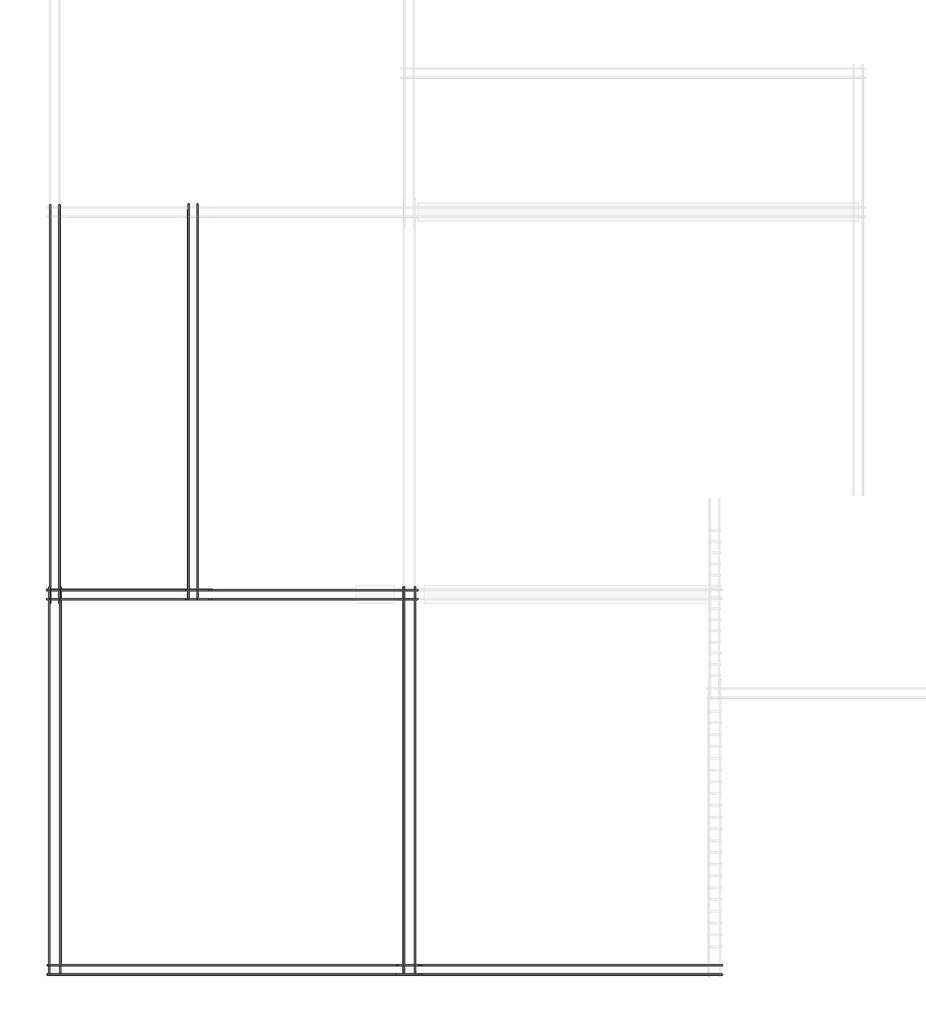
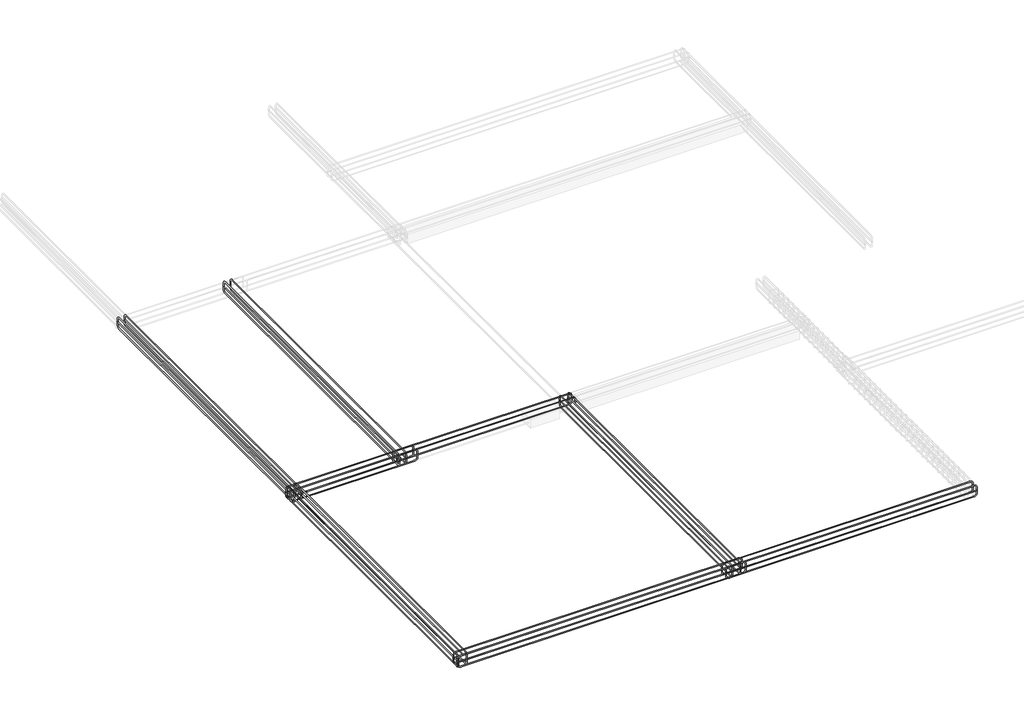
# One storey, part 2 of 5: 45 reinforcing bars.
"""IFC4 building model written with IfcOpenShell, lengths in millimetres."""

from ifc_helpers import new_model, si_unit, point, frame, origin, place, context, project, spatial, polyline, circle_curve, trimmed, segment, composite_curve, element, save
from ifc_brep_helpers import swept_disk

model = new_model("IFC4")

# Units and contexts
model_context = context("Model", 3, world=origin())
ifc_project = project(units=[si_unit("LENGTHUNIT", "METRE", prefix="MILLI")], contexts=[model_context])

# Site, building, storey
site = spatial("IfcSite", under=ifc_project)
building = spatial("IfcBuilding", under=site)
storey = spatial("IfcBuildingStorey", under=building, Elevation=0.0)

# Reinforcing bars
placement = place(None, origin())
element("IfcReinforcingBar", 1, at=placement, inside=storey, context=model_context, shape_type="SolidModel", body=[
    swept_disk(composite_curve([segment(polyline([(-14810.5016244, 4871.519882, 304.2552561), (-14810.5016244, 4871.519882, 355.0552561)]), True, "CONTINUOUS"), segment(trimmed(circle_curve(frame((-14766.0516244, 4871.519882, 355.0552561), z_axis=(0.0, 1.0, 0.0), x_axis=(-44.45000000000073, 0.0, 0.0)), 44.45), [point((-14810.5016244, 4871.519882, 355.0552561))], [point((-14766.0516244, 4871.519882, 399.5052561))], True, "CARTESIAN"), True, "CONTINUOUS"), segment(polyline([(-14766.0516244, 4871.519882, 399.5052561), (-12753.7926107, 4871.519882, 399.5052561)]), True, "CONTINUOUS"), segment(trimmed(circle_curve(frame((-12753.7926107, 4871.519882, 355.0552561), z_axis=(0.0, 1.0, 0.0), x_axis=(0.0, 0.0, 44.44999999999999)), 44.45), [point((-12753.7926107, 4871.519882, 399.5052561))], [point((-12709.3426107, 4871.519882, 355.0552561))], True, "CARTESIAN"), True, "CONTINUOUS"), segment(polyline([(-12709.3426107, 4871.519882, 355.0552561), (-12709.3426107, 4871.519882, 304.2552561)]), True, "CONTINUOUS")], self_intersect=False), 6.35),
])
element("IfcReinforcingBar", 2, at=placement, inside=storey, context=model_context, shape_type="SolidModel", body=[
    swept_disk(composite_curve([segment(polyline([(-14811.119206, 4984.7303943, 304.2552561), (-14811.119206, 4984.7303943, 355.0552561)]), True, "CONTINUOUS"), segment(trimmed(circle_curve(frame((-14766.669206, 4984.7303943, 355.0552561), z_axis=(0.0, 1.0, 0.0), x_axis=(-44.44999999999891, 0.0, 0.0)), 44.45), [point((-14811.119206, 4984.7303943, 355.0552561))], [point((-14766.669206, 4984.7303943, 399.5052561))], True, "CARTESIAN"), True, "CONTINUOUS"), segment(polyline([(-14766.669206, 4984.7303943, 399.5052561), (-12753.8888906, 4984.7303943, 399.5052561)]), True, "CONTINUOUS"), segment(trimmed(circle_curve(frame((-12753.8888906, 4984.7303943, 355.0552561), z_axis=(0.0, 1.0, 0.0), x_axis=(0.0, 0.0, 44.44999999999999)), 44.45), [point((-12753.8888906, 4984.7303943, 399.5052561))], [point((-12709.4388906, 4984.7303943, 355.0552561))], True, "CARTESIAN"), True, "CONTINUOUS"), segment(polyline([(-12709.4388906, 4984.7303943, 355.0552561), (-12709.4388906, 4984.7303943, 304.2552561)]), True, "CONTINUOUS")], self_intersect=False), 6.35),
])
element("IfcReinforcingBar", 3, at=placement, inside=storey, context=model_context, shape_type="SolidModel", body=[
    swept_disk(composite_curve([segment(polyline([(-14810.6974131, 4871.519882, 305.3447439), (-14810.6974131, 4871.519882, 254.5447439)]), True, "CONTINUOUS"), segment(trimmed(circle_curve(frame((-14766.2474131, 4871.519882, 254.5447439), z_axis=(0.0, -1.0, 0.0), x_axis=(-44.45000000000073, 0.0, 0.0)), 44.45), [point((-14810.6974131, 4871.519882, 254.5447439))], [point((-14766.2474131, 4871.519882, 210.0947439))], True, "CARTESIAN"), True, "CONTINUOUS"), segment(polyline([(-14766.2474131, 4871.519882, 210.0947439), (-12754.044612, 4871.519882, 210.0947439)]), True, "CONTINUOUS"), segment(trimmed(circle_curve(frame((-12754.044612, 4871.519882, 254.5447439), z_axis=(0.0, -1.0, 0.0), x_axis=(0.0, 0.0, -44.44999999999999)), 44.45), [point((-12754.044612, 4871.519882, 210.0947439))], [point((-12709.594612, 4871.519882, 254.5447439))], True, "CARTESIAN"), True, "CONTINUOUS"), segment(polyline([(-12709.594612, 4871.519882, 254.5447439), (-12709.594612, 4871.519882, 305.3447439)]), True, "CONTINUOUS")], self_intersect=False), 6.35),
])
element("IfcReinforcingBar", 4, at=placement, inside=storey, context=model_context, shape_type="SolidModel", body=[
    swept_disk(composite_curve([segment(polyline([(-14812.0419124, 4984.7303943, 305.3447439), (-14812.0419124, 4984.7303943, 254.5447439)]), True, "CONTINUOUS"), segment(trimmed(circle_curve(frame((-14767.5919124, 4984.7303943, 254.5447439), z_axis=(0.0, -1.0, 0.0), x_axis=(-44.45000000000073, 0.0, 0.0)), 44.45), [point((-14812.0419124, 4984.7303943, 254.5447439))], [point((-14767.5919124, 4984.7303943, 210.0947439))], True, "CARTESIAN"), True, "CONTINUOUS"), segment(polyline([(-14767.5919124, 4984.7303943, 210.0947439), (-12754.4128441, 4984.7303943, 210.0947439)]), True, "CONTINUOUS"), segment(trimmed(circle_curve(frame((-12754.4128441, 4984.7303943, 254.5447439), z_axis=(0.0, -1.0, 0.0), x_axis=(0.0, 0.0, -44.44999999999999)), 44.45), [point((-12754.4128441, 4984.7303943, 210.0947439))], [point((-12709.9628441, 4984.7303943, 254.5447439))], True, "CARTESIAN"), True, "CONTINUOUS"), segment(polyline([(-12709.9628441, 4984.7303943, 254.5447439), (-12709.9628441, 4984.7303943, 305.3447439)]), True, "CONTINUOUS")], self_intersect=False), 6.35),
])
element("IfcReinforcingBar", 5, at=placement, inside=storey, context=model_context, shape_type="SolidModel", body=[
    swept_disk(composite_curve([segment(polyline([(-14534.7918223, 4867.8001382, 304.8), (-13131.4418223, 4867.8001382, 304.8)]), True, "CONTINUOUS")], self_intersect=False), 6.35),
])
element("IfcReinforcingBar", 6, at=placement, inside=storey, context=model_context, shape_type="SolidModel", body=[
    swept_disk(composite_curve([segment(polyline([(-14818.480298, 4988.4501382, 304.8), (-12703.1933611, 4988.4501382, 304.8)]), True, "CONTINUOUS")], self_intersect=False), 6.35),
])
element("IfcReinforcingBar", 7, at=placement, inside=storey, context=model_context, shape_type="SolidModel", body=[
    swept_disk(composite_curve([segment(polyline([(-10097.104427, 4984.7303943, 304.2552561), (-10097.104427, 4984.7303943, 355.0552561)]), True, "CONTINUOUS"), segment(trimmed(circle_curve(frame((-10141.554427, 4984.7303943, 355.0552561), z_axis=(0.0, -1.0, 0.0), x_axis=(44.44999999999891, 0.0, 0.0)), 44.45), [point((-10097.104427, 4984.7303943, 355.0552561))], [point((-10141.554427, 4984.7303943, 399.5052561))], True, "CARTESIAN"), True, "CONTINUOUS"), segment(polyline([(-10141.554427, 4984.7303943, 399.5052561), (-13001.0910339, 4984.7303943, 399.5052561)]), True, "CONTINUOUS"), segment(trimmed(circle_curve(frame((-13001.0910339, 4984.7303943, 355.0552561), z_axis=(0.0, -1.0, 0.0), x_axis=(0.0, 0.0, 44.44999999999999)), 44.45), [point((-13001.0910339, 4984.7303943, 399.5052561))], [point((-13045.5410339, 4984.7303943, 355.0552561))], True, "CARTESIAN"), True, "CONTINUOUS"), segment(polyline([(-13045.5410339, 4984.7303943, 355.0552561), (-13045.5410339, 4984.7303943, 304.2552561)]), True, "CONTINUOUS")], self_intersect=False), 6.35),
])
element("IfcReinforcingBar", 8, at=placement, inside=storey, context=model_context, shape_type="SolidModel", body=[
    swept_disk(composite_curve([segment(polyline([(-10097.5426731, 4871.519882, 304.2552561), (-10097.5426731, 4871.519882, 355.0552561)]), True, "CONTINUOUS"), segment(trimmed(circle_curve(frame((-10141.9926731, 4871.519882, 355.0552561), z_axis=(0.0, -1.0, 0.0), x_axis=(44.44999999999891, 0.0, 0.0)), 44.45), [point((-10097.5426731, 4871.519882, 355.0552561))], [point((-10141.9926731, 4871.519882, 399.5052561))], True, "CARTESIAN"), True, "CONTINUOUS"), segment(polyline([(-10141.9926731, 4871.519882, 399.5052561), (-13000.994754, 4871.519882, 399.5052561)]), True, "CONTINUOUS"), segment(trimmed(circle_curve(frame((-13000.994754, 4871.519882, 355.0552561), z_axis=(0.0, -1.0, 0.0), x_axis=(0.0, 0.0, 44.44999999999999)), 44.45), [point((-13000.994754, 4871.519882, 399.5052561))], [point((-13045.444754, 4871.519882, 355.0552561))], True, "CARTESIAN"), True, "CONTINUOUS"), segment(polyline([(-13045.444754, 4871.519882, 355.0552561), (-13045.444754, 4871.519882, 304.2552561)]), True, "CONTINUOUS")], self_intersect=False), 6.35),
])
element("IfcReinforcingBar", 9, at=placement, inside=storey, context=model_context, shape_type="SolidModel", body=[
    swept_disk(composite_curve([segment(polyline([(-10095.8402778, 4984.7303943, 305.3447439), (-10095.8402778, 4984.7303943, 254.5447439)]), True, "CONTINUOUS"), segment(trimmed(circle_curve(frame((-10140.2902778, 4984.7303943, 254.5447439), z_axis=(0.0, 1.0, 0.0), x_axis=(44.45000000000073, 0.0, 0.0)), 44.45), [point((-10095.8402778, 4984.7303943, 254.5447439))], [point((-10140.2902778, 4984.7303943, 210.0947439))], True, "CARTESIAN"), True, "CONTINUOUS"), segment(polyline([(-10140.2902778, 4984.7303943, 210.0947439), (-13000.8390327, 4984.7303943, 210.0947439)]), True, "CONTINUOUS"), segment(trimmed(circle_curve(frame((-13000.8390327, 4984.7303943, 254.5447439), z_axis=(0.0, 1.0, 0.0), x_axis=(0.0, 0.0, -44.44999999999999)), 44.45), [point((-13000.8390327, 4984.7303943, 210.0947439))], [point((-13045.2890327, 4984.7303943, 254.5447439))], True, "CARTESIAN"), True, "CONTINUOUS"), segment(polyline([(-13045.2890327, 4984.7303943, 254.5447439), (-13045.2890327, 4984.7303943, 305.3447439)]), True, "CONTINUOUS")], self_intersect=False), 6.35),
])
element("IfcReinforcingBar", 10, at=placement, inside=storey, context=model_context, shape_type="SolidModel", body=[
    swept_disk(composite_curve([segment(polyline([(-6221.7854997, 209.9629274, 304.2552561), (-6221.7854997, 209.9629274, 355.0552561)]), True, "CONTINUOUS"), segment(trimmed(circle_curve(frame((-6266.2354997, 209.9629274, 355.0552561), z_axis=(0.0, -1.0, 0.0), x_axis=(44.44999999999982, 0.0, 0.0)), 44.45), [point((-6221.7854997, 209.9629274, 355.0552561))], [point((-6266.2354997, 209.9629274, 399.5052561))], True, "CARTESIAN"), True, "CONTINUOUS"), segment(polyline([(-6266.2354997, 209.9629274, 399.5052561), (-10321.3910339, 209.9629274, 399.5052561)]), True, "CONTINUOUS"), segment(trimmed(circle_curve(frame((-10321.3910339, 209.9629274, 355.0552561), z_axis=(0.0, -1.0, 0.0), x_axis=(0.0, 0.0, 44.44999999999999)), 44.45), [point((-10321.3910339, 209.9629274, 399.5052561))], [point((-10365.8410339, 209.9629274, 355.0552561))], True, "CARTESIAN"), True, "CONTINUOUS"), segment(polyline([(-10365.8410339, 209.9629274, 355.0552561), (-10365.8410339, 209.9629274, 304.2552561)]), True, "CONTINUOUS")], self_intersect=False), 6.35),
])
element("IfcReinforcingBar", 11, at=placement, inside=storey, context=model_context, shape_type="SolidModel", body=[
    swept_disk(composite_curve([segment(polyline([(-6222.3875013, 96.7524151, 304.2552561), (-6222.3875013, 96.7524151, 355.0552561)]), True, "CONTINUOUS"), segment(trimmed(circle_curve(frame((-6266.8375013, 96.7524151, 355.0552561), z_axis=(0.0, -1.0, 0.0), x_axis=(44.45000000000073, 0.0, 0.0)), 44.45), [point((-6222.3875013, 96.7524151, 355.0552561))], [point((-6266.8375013, 96.7524151, 399.5052561))], True, "CARTESIAN"), True, "CONTINUOUS"), segment(polyline([(-6266.8375013, 96.7524151, 399.5052561), (-10321.294754, 96.7524151, 399.5052561)]), True, "CONTINUOUS"), segment(trimmed(circle_curve(frame((-10321.294754, 96.7524151, 355.0552561), z_axis=(0.0, -1.0, 0.0), x_axis=(0.0, 0.0, 44.44999999999999)), 44.45), [point((-10321.294754, 96.7524151, 399.5052561))], [point((-10365.744754, 96.7524151, 355.0552561))], True, "CARTESIAN"), True, "CONTINUOUS"), segment(polyline([(-10365.744754, 96.7524151, 355.0552561), (-10365.744754, 96.7524151, 304.2552561)]), True, "CONTINUOUS")], self_intersect=False), 6.35),
])
element("IfcReinforcingBar", 12, at=placement, inside=storey, context=model_context, shape_type="SolidModel", body=[
    swept_disk(composite_curve([segment(polyline([(-6222.9639641, 209.9629274, 305.3447439), (-6222.9639641, 209.9629274, 254.5447439)]), True, "CONTINUOUS"), segment(trimmed(circle_curve(frame((-6267.4139641, 209.9629274, 254.5447439), z_axis=(0.0, 1.0, 0.0), x_axis=(44.44999999999982, 0.0, 0.0)), 44.45), [point((-6222.9639641, 209.9629274, 254.5447439))], [point((-6267.4139641, 209.9629274, 210.0947439))], True, "CARTESIAN"), True, "CONTINUOUS"), segment(polyline([(-6267.4139641, 209.9629274, 210.0947439), (-10321.1390327, 209.9629274, 210.0947439)]), True, "CONTINUOUS"), segment(trimmed(circle_curve(frame((-10321.1390327, 209.9629274, 254.5447439), z_axis=(0.0, 1.0, 0.0), x_axis=(0.0, 0.0, -44.44999999999999)), 44.45), [point((-10321.1390327, 209.9629274, 210.0947439))], [point((-10365.5890327, 209.9629274, 254.5447439))], True, "CARTESIAN"), True, "CONTINUOUS"), segment(polyline([(-10365.5890327, 209.9629274, 254.5447439), (-10365.5890327, 209.9629274, 305.3447439)]), True, "CONTINUOUS")], self_intersect=False), 6.35),
])
element("IfcReinforcingBar", 13, at=placement, inside=storey, context=model_context, shape_type="SolidModel", body=[
    swept_disk(composite_curve([segment(polyline([(-6223.2425489, 96.7524151, 305.3447439), (-6223.2425489, 96.7524151, 254.5447439)]), True, "CONTINUOUS"), segment(trimmed(circle_curve(frame((-6267.6925489, 96.7524151, 254.5447439), z_axis=(0.0, 1.0, 0.0), x_axis=(44.44999999999982, 0.0, 0.0)), 44.45), [point((-6223.2425489, 96.7524151, 254.5447439))], [point((-6267.6925489, 96.7524151, 210.0947439))], True, "CARTESIAN"), True, "CONTINUOUS"), segment(polyline([(-6267.6925489, 96.7524151, 210.0947439), (-10320.7708006, 96.7524151, 210.0947439)]), True, "CONTINUOUS"), segment(trimmed(circle_curve(frame((-10320.7708006, 96.7524151, 254.5447439), z_axis=(0.0, 1.0, 0.0), x_axis=(0.0, 0.0, -44.44999999999999)), 44.45), [point((-10320.7708006, 96.7524151, 210.0947439))], [point((-10365.2208006, 96.7524151, 254.5447439))], True, "CARTESIAN"), True, "CONTINUOUS"), segment(polyline([(-10365.2208006, 96.7524151, 254.5447439), (-10365.2208006, 96.7524151, 305.3447439)]), True, "CONTINUOUS")], self_intersect=False), 6.35),
])
element("IfcReinforcingBar", 14, at=placement, inside=storey, context=model_context, shape_type="SolidModel", body=[
    swept_disk(composite_curve([segment(polyline([(-6216.0848989, 213.6826713, 304.8), (-10311.3420725, 213.6826713, 304.8)]), True, "CONTINUOUS")], self_intersect=False), 6.35),
])
element("IfcReinforcingBar", 15, at=placement, inside=storey, context=model_context, shape_type="SolidModel", body=[
    swept_disk(composite_curve([segment(polyline([(-6215.9707513, 93.0326713, 304.8), (-10371.9902836, 93.0326713, 304.8)]), True, "CONTINUOUS")], self_intersect=False), 6.35),
])
element("IfcReinforcingBar", 16, at=placement, inside=storey, context=model_context, shape_type="SolidModel", body=[
    swept_disk(composite_curve([segment(polyline([(-10040.6958382, 209.9629274, 304.2552561), (-10040.6958382, 209.9629274, 355.0552561)]), True, "CONTINUOUS"), segment(trimmed(circle_curve(frame((-10085.1458382, 209.9629274, 355.0552561), z_axis=(0.0, -1.0, 0.0), x_axis=(44.45000000000073, 0.0, 0.0)), 44.45), [point((-10040.6958382, 209.9629274, 355.0552561))], [point((-10085.1458382, 209.9629274, 399.5052561))], True, "CARTESIAN"), True, "CONTINUOUS"), segment(polyline([(-10085.1458382, 209.9629274, 399.5052561), (-14760.0410339, 209.9629274, 399.5052561)]), True, "CONTINUOUS"), segment(trimmed(circle_curve(frame((-14760.0410339, 209.9629274, 355.0552561), z_axis=(0.0, -1.0, 0.0), x_axis=(0.0, 0.0, 44.44999999999999)), 44.45), [point((-14760.0410339, 209.9629274, 399.5052561))], [point((-14804.4910339, 209.9629274, 355.0552561))], True, "CARTESIAN"), True, "CONTINUOUS"), segment(polyline([(-14804.4910339, 209.9629274, 355.0552561), (-14804.4910339, 209.9629274, 304.2552561)]), True, "CONTINUOUS")], self_intersect=False), 6.35),
])
element("IfcReinforcingBar", 17, at=placement, inside=storey, context=model_context, shape_type="SolidModel", body=[
    swept_disk(composite_curve([segment(polyline([(-10040.7832995, 96.7524151, 304.2552561), (-10040.7832995, 96.7524151, 355.0552561)]), True, "CONTINUOUS"), segment(trimmed(circle_curve(frame((-10085.2332995, 96.7524151, 355.0552561), z_axis=(0.0, -1.0, 0.0), x_axis=(44.44999999999891, 0.0, 0.0)), 44.45), [point((-10040.7832995, 96.7524151, 355.0552561))], [point((-10085.2332995, 96.7524151, 399.5052561))], True, "CARTESIAN"), True, "CONTINUOUS"), segment(polyline([(-10085.2332995, 96.7524151, 399.5052561), (-14759.944754, 96.7524151, 399.5052561)]), True, "CONTINUOUS"), segment(trimmed(circle_curve(frame((-14759.944754, 96.7524151, 355.0552561), z_axis=(0.0, -1.0, 0.0), x_axis=(0.0, 0.0, 44.44999999999999)), 44.45), [point((-14759.944754, 96.7524151, 399.5052561))], [point((-14804.394754, 96.7524151, 355.0552561))], True, "CARTESIAN"), True, "CONTINUOUS"), segment(polyline([(-14804.394754, 96.7524151, 355.0552561), (-14804.394754, 96.7524151, 304.2552561)]), True, "CONTINUOUS")], self_intersect=False), 6.35),
])
element("IfcReinforcingBar", 18, at=placement, inside=storey, context=model_context, shape_type="SolidModel", body=[
    swept_disk(composite_curve([segment(polyline([(-10042.0160096, 209.9629274, 305.3447439), (-10042.0160096, 209.9629274, 254.5447439)]), True, "CONTINUOUS"), segment(trimmed(circle_curve(frame((-10086.4660096, 209.9629274, 254.5447439), z_axis=(0.0, 1.0, 0.0), x_axis=(44.45000000000073, 0.0, 0.0)), 44.45), [point((-10042.0160096, 209.9629274, 254.5447439))], [point((-10086.4660096, 209.9629274, 210.0947439))], True, "CARTESIAN"), True, "CONTINUOUS"), segment(polyline([(-10086.4660096, 209.9629274, 210.0947439), (-14759.7890327, 209.9629274, 210.0947439)]), True, "CONTINUOUS"), segment(trimmed(circle_curve(frame((-14759.7890327, 209.9629274, 254.5447439), z_axis=(0.0, 1.0, 0.0), x_axis=(0.0, 0.0, -44.44999999999999)), 44.45), [point((-14759.7890327, 209.9629274, 210.0947439))], [point((-14804.2390327, 209.9629274, 254.5447439))], True, "CARTESIAN"), True, "CONTINUOUS"), segment(polyline([(-14804.2390327, 209.9629274, 254.5447439), (-14804.2390327, 209.9629274, 305.3447439)]), True, "CONTINUOUS")], self_intersect=False), 6.35),
])
element("IfcReinforcingBar", 19, at=placement, inside=storey, context=model_context, shape_type="SolidModel", body=[
    swept_disk(composite_curve([segment(polyline([(-10041.3559239, 96.7524151, 305.3447439), (-10041.3559239, 96.7524151, 254.5447439)]), True, "CONTINUOUS"), segment(trimmed(circle_curve(frame((-10085.8059239, 96.7524151, 254.5447439), z_axis=(0.0, 1.0, 0.0), x_axis=(44.44999999999891, 0.0, 0.0)), 44.45), [point((-10041.3559239, 96.7524151, 254.5447439))], [point((-10085.8059239, 96.7524151, 210.0947439))], True, "CARTESIAN"), True, "CONTINUOUS"), segment(polyline([(-10085.8059239, 96.7524151, 210.0947439), (-14759.4208006, 96.7524151, 210.0947439)]), True, "CONTINUOUS"), segment(trimmed(circle_curve(frame((-14759.4208006, 96.7524151, 254.5447439), z_axis=(0.0, 1.0, 0.0), x_axis=(0.0, 0.0, -44.44999999999999)), 44.45), [point((-14759.4208006, 96.7524151, 210.0947439))], [point((-14803.8708006, 96.7524151, 254.5447439))], True, "CARTESIAN"), True, "CONTINUOUS"), segment(polyline([(-14803.8708006, 96.7524151, 254.5447439), (-14803.8708006, 96.7524151, 305.3447439)]), True, "CONTINUOUS")], self_intersect=False), 6.35),
])
element("IfcReinforcingBar", 20, at=placement, inside=storey, context=model_context, shape_type="SolidModel", body=[
    swept_disk(composite_curve([segment(polyline([(-10084.5322341, 213.6826713, 304.8), (-14809.5352998, 213.6826713, 304.8)]), True, "CONTINUOUS")], self_intersect=False), 6.35),
])
element("IfcReinforcingBar", 21, at=placement, inside=storey, context=model_context, shape_type="SolidModel", body=[
    swept_disk(composite_curve([segment(polyline([(-10086.4986582, 93.0326713, 304.8), (-14810.6402836, 93.0326713, 304.8)]), True, "CONTINUOUS")], self_intersect=False), 6.35),
])
element("IfcReinforcingBar", 22, at=placement, inside=storey, context=model_context, shape_type="SolidModel", body=[
    swept_disk(composite_curve([segment(polyline([(-10128.4365662, 92.8452695, 304.2552561), (-10128.4365662, 92.8452695, 355.0552561)]), True, "CONTINUOUS"), segment(trimmed(circle_curve(frame((-10128.4365662, 137.2952695, 355.0552561), z_axis=(-1.0, 0.0, 0.0), x_axis=(0.0, -44.44999999999999, 0.0)), 44.45), [point((-10128.4365662, 92.8452695, 355.0552561))], [point((-10128.4365662, 137.2952695, 399.5052561))], True, "CARTESIAN"), True, "CONTINUOUS"), segment(polyline([(-10128.4365662, 137.2952695, 399.5052561), (-10128.4365662, 4977.1529731, 399.5052561)]), True, "CONTINUOUS"), segment(trimmed(circle_curve(frame((-10128.4365662, 4977.1529731, 355.0552561), z_axis=(-1.0, 0.0, 0.0), x_axis=(0.0, 0.0, 44.44999999999999)), 44.45), [point((-10128.4365662, 4977.1529731, 399.5052561))], [point((-10128.4365662, 5021.6029731, 355.0552561))], True, "CARTESIAN"), True, "CONTINUOUS"), segment(polyline([(-10128.4365662, 5021.6029731, 355.0552561), (-10128.4365662, 5021.6029731, 304.2552561)]), True, "CONTINUOUS")], self_intersect=False), 6.35),
])
element("IfcReinforcingBar", 23, at=placement, inside=storey, context=model_context, shape_type="SolidModel", body=[
    swept_disk(composite_curve([segment(polyline([(-10267.0470784, 92.9792716, 304.2552561), (-10267.0470784, 92.9792716, 355.0552561)]), True, "CONTINUOUS"), segment(trimmed(circle_curve(frame((-10267.0470784, 137.4292716, 355.0552561), z_axis=(-1.0, 0.0, 0.0), x_axis=(0.0, -44.44999999999999, 0.0)), 44.45), [point((-10267.0470784, 92.9792716, 355.0552561))], [point((-10267.0470784, 137.4292716, 399.5052561))], True, "CARTESIAN"), True, "CONTINUOUS"), segment(polyline([(-10267.0470784, 137.4292716, 399.5052561), (-10267.0470784, 4977.0498865, 399.5052561)]), True, "CONTINUOUS"), segment(trimmed(circle_curve(frame((-10267.0470784, 4977.0498865, 355.0552561), z_axis=(-1.0, 0.0, 0.0), x_axis=(0.0, 0.0, 44.44999999999999)), 44.45), [point((-10267.0470784, 4977.0498865, 399.5052561))], [point((-10267.0470784, 5021.4998865, 355.0552561))], True, "CARTESIAN"), True, "CONTINUOUS"), segment(polyline([(-10267.0470784, 5021.4998865, 355.0552561), (-10267.0470784, 5021.4998865, 304.2552561)]), True, "CONTINUOUS")], self_intersect=False), 6.35),
])
element("IfcReinforcingBar", 24, at=placement, inside=storey, context=model_context, shape_type="SolidModel", body=[
    swept_disk(composite_curve([segment(polyline([(-10128.4365662, 93.5768417, 292.6447439), (-10128.4365662, 93.5768417, 241.8447439)]), True, "CONTINUOUS"), segment(trimmed(circle_curve(frame((-10128.4365662, 138.0268417, 241.8447439), z_axis=(1.0, 0.0, 0.0), x_axis=(0.0, -44.45, 0.0)), 44.45), [point((-10128.4365662, 93.5768417, 241.8447439))], [point((-10128.4365662, 138.0268417, 197.3947439))], True, "CARTESIAN"), True, "CONTINUOUS"), segment(polyline([(-10128.4365662, 138.0268417, 197.3947439), (-10128.4365662, 4976.4997012, 197.3947439)]), True, "CONTINUOUS"), segment(trimmed(circle_curve(frame((-10128.4365662, 4976.4997012, 241.8447439), z_axis=(1.0, 0.0, 0.0), x_axis=(0.0, 0.0, -44.44999999999999)), 44.45), [point((-10128.4365662, 4976.4997012, 197.3947439))], [point((-10128.4365662, 5020.9497012, 241.8447439))], True, "CARTESIAN"), True, "CONTINUOUS"), segment(polyline([(-10128.4365662, 5020.9497012, 241.8447439), (-10128.4365662, 5020.9497012, 292.6447439)]), True, "CONTINUOUS")], self_intersect=False), 6.35),
])
element("IfcReinforcingBar", 25, at=placement, inside=storey, context=model_context, shape_type="SolidModel", body=[
    swept_disk(composite_curve([segment(polyline([(-10267.0470784, 93.8151458, 292.6447439), (-10267.0470784, 93.8151458, 241.8447439)]), True, "CONTINUOUS"), segment(trimmed(circle_curve(frame((-10267.0470784, 138.2651458, 241.8447439), z_axis=(1.0, 0.0, 0.0), x_axis=(0.0, -44.45, 0.0)), 44.45), [point((-10267.0470784, 93.8151458, 241.8447439))], [point((-10267.0470784, 138.2651458, 197.3947439))], True, "CARTESIAN"), True, "CONTINUOUS"), segment(polyline([(-10267.0470784, 138.2651458, 197.3947439), (-10267.0470784, 4976.5301582, 197.3947439)]), True, "CONTINUOUS"), segment(trimmed(circle_curve(frame((-10267.0470784, 4976.5301582, 241.8447439), z_axis=(1.0, 0.0, 0.0), x_axis=(0.0, 0.0, -44.44999999999999)), 44.45), [point((-10267.0470784, 4976.5301582, 197.3947439))], [point((-10267.0470784, 5020.9801582, 241.8447439))], True, "CARTESIAN"), True, "CONTINUOUS"), segment(polyline([(-10267.0470784, 5020.9801582, 241.8447439), (-10267.0470784, 5020.9801582, 292.6447439)]), True, "CONTINUOUS")], self_intersect=False), 6.35),
])
element("IfcReinforcingBar", 26, at=placement, inside=storey, context=model_context, shape_type="SolidModel", body=[
    swept_disk(composite_curve([segment(polyline([(-10124.7168223, 86.8753425, 304.8), (-10124.7168223, 5028.0332844, 304.8)]), True, "CONTINUOUS")], self_intersect=False), 6.35),
])
element("IfcReinforcingBar", 27, at=placement, inside=storey, context=model_context, shape_type="SolidModel", body=[
    swept_disk(composite_curve([segment(polyline([(-10270.7668223, 87.0104308, 304.8), (-10270.7668223, 5028.0628813, 304.8)]), True, "CONTINUOUS")], self_intersect=False), 6.35),
])
element("IfcReinforcingBar", 28, at=placement, inside=storey, context=model_context, shape_type="SolidModel", body=[
    swept_disk(composite_curve([segment(polyline([(-14781.8970784, 5017.8814608, 304.2552561), (-14781.8970784, 5017.8814608, 355.0552561)]), True, "CONTINUOUS"), segment(trimmed(circle_curve(frame((-14781.8970784, 4973.4314608, 355.0552561), z_axis=(1.0, 0.0, 0.0), x_axis=(0.0, 44.44999999999982, 0.0)), 44.45), [point((-14781.8970784, 5017.8814608, 355.0552561))], [point((-14781.8970784, 4973.4314608, 399.5052561))], True, "CARTESIAN"), True, "CONTINUOUS"), segment(polyline([(-14781.8970784, 4973.4314608, 399.5052561), (-14781.8970784, 148.2539748, 399.5052561)]), True, "CONTINUOUS"), segment(trimmed(circle_curve(frame((-14781.8970784, 148.2539748, 355.0552561), z_axis=(1.0, 0.0, 0.0), x_axis=(0.0, 0.0, 44.44999999999999)), 44.45), [point((-14781.8970784, 148.2539748, 399.5052561))], [point((-14781.8970784, 103.8039748, 355.0552561))], True, "CARTESIAN"), True, "CONTINUOUS"), segment(polyline([(-14781.8970784, 103.8039748, 355.0552561), (-14781.8970784, 103.8039748, 304.2552561)]), True, "CONTINUOUS")], self_intersect=False), 6.35),
])
element("IfcReinforcingBar", 29, at=placement, inside=storey, context=model_context, shape_type="SolidModel", body=[
    swept_disk(composite_curve([segment(polyline([(-14643.2865662, 5017.2794592, 304.2552561), (-14643.2865662, 5017.2794592, 355.0552561)]), True, "CONTINUOUS"), segment(trimmed(circle_curve(frame((-14643.2865662, 4972.8294592, 355.0552561), z_axis=(1.0, 0.0, 0.0), x_axis=(0.0, 44.44999999999982, 0.0)), 44.45), [point((-14643.2865662, 5017.2794592, 355.0552561))], [point((-14643.2865662, 4972.8294592, 399.5052561))], True, "CARTESIAN"), True, "CONTINUOUS"), segment(polyline([(-14643.2865662, 4972.8294592, 399.5052561), (-14643.2865662, 147.8756109, 399.5052561)]), True, "CONTINUOUS"), segment(trimmed(circle_curve(frame((-14643.2865662, 147.8756109, 355.0552561), z_axis=(1.0, 0.0, 0.0), x_axis=(0.0, 0.0, 44.44999999999999)), 44.45), [point((-14643.2865662, 147.8756109, 399.5052561))], [point((-14643.2865662, 103.4256109, 355.0552561))], True, "CARTESIAN"), True, "CONTINUOUS"), segment(polyline([(-14643.2865662, 103.4256109, 355.0552561), (-14643.2865662, 103.4256109, 304.2552561)]), True, "CONTINUOUS")], self_intersect=False), 6.35),
])
element("IfcReinforcingBar", 30, at=placement, inside=storey, context=model_context, shape_type="SolidModel", body=[
    swept_disk(composite_curve([segment(polyline([(-14781.8970784, 5016.7029964, 292.6447439), (-14781.8970784, 5016.7029964, 241.8447439)]), True, "CONTINUOUS"), segment(trimmed(circle_curve(frame((-14781.8970784, 4972.2529964, 241.8447439), z_axis=(-1.0, 0.0, 0.0), x_axis=(0.0, 44.45000000000073, 0.0)), 44.45), [point((-14781.8970784, 5016.7029964, 241.8447439))], [point((-14781.8970784, 4972.2529964, 197.3947439))], True, "CARTESIAN"), True, "CONTINUOUS"), segment(polyline([(-14781.8970784, 4972.2529964, 197.3947439), (-14781.8970784, 148.3049496, 197.3947439)]), True, "CONTINUOUS"), segment(trimmed(circle_curve(frame((-14781.8970784, 148.3049496, 241.8447439), z_axis=(-1.0, 0.0, 0.0), x_axis=(0.0, 0.0, -44.44999999999999)), 44.45), [point((-14781.8970784, 148.3049496, 197.3947439))], [point((-14781.8970784, 103.8549496, 241.8447439))], True, "CARTESIAN"), True, "CONTINUOUS"), segment(polyline([(-14781.8970784, 103.8549496, 241.8447439), (-14781.8970784, 103.8549496, 292.6447439)]), True, "CONTINUOUS")], self_intersect=False), 6.35),
])
element("IfcReinforcingBar", 31, at=placement, inside=storey, context=model_context, shape_type="SolidModel", body=[
    swept_disk(composite_curve([segment(polyline([(-14643.2865662, 5016.4244116, 292.6447439), (-14643.2865662, 5016.4244116, 241.8447439)]), True, "CONTINUOUS"), segment(trimmed(circle_curve(frame((-14643.2865662, 4971.9744116, 241.8447439), z_axis=(-1.0, 0.0, 0.0), x_axis=(0.0, 44.44999999999982, 0.0)), 44.45), [point((-14643.2865662, 5016.4244116, 241.8447439))], [point((-14643.2865662, 4971.9744116, 197.3947439))], True, "CARTESIAN"), True, "CONTINUOUS"), segment(polyline([(-14643.2865662, 4971.9744116, 197.3947439), (-14643.2865662, 148.0409303, 197.3947439)]), True, "CONTINUOUS"), segment(trimmed(circle_curve(frame((-14643.2865662, 148.0409303, 241.8447439), z_axis=(-1.0, 0.0, 0.0), x_axis=(0.0, 0.0, -44.44999999999999)), 44.45), [point((-14643.2865662, 148.0409303, 197.3947439))], [point((-14643.2865662, 103.5909303, 241.8447439))], True, "CARTESIAN"), True, "CONTINUOUS"), segment(polyline([(-14643.2865662, 103.5909303, 241.8447439), (-14643.2865662, 103.5909303, 292.6447439)]), True, "CONTINUOUS")], self_intersect=False), 6.35),
])
element("IfcReinforcingBar", 32, at=placement, inside=storey, context=model_context, shape_type="SolidModel", body=[
    swept_disk(composite_curve([segment(polyline([(-14785.6168223, 5023.5820616, 304.8), (-14785.6168223, 94.7861956, 304.8)]), True, "CONTINUOUS")], self_intersect=False), 6.35),
])
element("IfcReinforcingBar", 33, at=placement, inside=storey, context=model_context, shape_type="SolidModel", body=[
    swept_disk(composite_curve([segment(polyline([(-14639.5668223, 5023.6962092, 304.8), (-14639.5668223, 236.062415, 304.8)]), True, "CONTINUOUS")], self_intersect=False), 6.35),
])
element("IfcReinforcingBar", 34, at=placement, inside=storey, context=model_context, shape_type="SolidModel", body=[
    swept_disk(composite_curve([segment(polyline([(-14769.1970784, 9882.4142028, 304.2552561), (-14769.1970784, 9882.4142028, 355.0552561)]), True, "CONTINUOUS"), segment(trimmed(circle_curve(frame((-14769.1970784, 9837.9642028, 355.0552561), z_axis=(1.0, 0.0, 0.0), x_axis=(0.0, 44.45000000000073, 0.0)), 44.45), [point((-14769.1970784, 9882.4142028, 355.0552561))], [point((-14769.1970784, 9837.9642028, 399.5052561))], True, "CARTESIAN"), True, "CONTINUOUS"), segment(polyline([(-14769.1970784, 9837.9642028, 399.5052561), (-14769.1970784, 4868.4086686, 399.5052561)]), True, "CONTINUOUS"), segment(trimmed(circle_curve(frame((-14769.1970784, 4868.4086686, 355.0552561), z_axis=(1.0, 0.0, 0.0), x_axis=(0.0, 0.0, 44.44999999999999)), 44.45), [point((-14769.1970784, 4868.4086686, 399.5052561))], [point((-14769.1970784, 4823.9586686, 355.0552561))], True, "CARTESIAN"), True, "CONTINUOUS"), segment(polyline([(-14769.1970784, 4823.9586686, 355.0552561), (-14769.1970784, 4823.9586686, 304.2552561)]), True, "CONTINUOUS")], self_intersect=False), 6.35),
])
element("IfcReinforcingBar", 35, at=placement, inside=storey, context=model_context, shape_type="SolidModel", body=[
    swept_disk(composite_curve([segment(polyline([(-14655.9865662, 9881.8122012, 304.2552561), (-14655.9865662, 9881.8122012, 355.0552561)]), True, "CONTINUOUS"), segment(trimmed(circle_curve(frame((-14655.9865662, 9837.3622012, 355.0552561), z_axis=(1.0, 0.0, 0.0), x_axis=(0.0, 44.45000000000073, 0.0)), 44.45), [point((-14655.9865662, 9881.8122012, 355.0552561))], [point((-14655.9865662, 9837.3622012, 399.5052561))], True, "CARTESIAN"), True, "CONTINUOUS"), segment(polyline([(-14655.9865662, 9837.3622012, 399.5052561), (-14655.9865662, 4868.5049485, 399.5052561)]), True, "CONTINUOUS"), segment(trimmed(circle_curve(frame((-14655.9865662, 4868.5049485, 355.0552561), z_axis=(1.0, 0.0, 0.0), x_axis=(0.0, 0.0, 44.44999999999999)), 44.45), [point((-14655.9865662, 4868.5049485, 399.5052561))], [point((-14655.9865662, 4824.0549485, 355.0552561))], True, "CARTESIAN"), True, "CONTINUOUS"), segment(polyline([(-14655.9865662, 4824.0549485, 355.0552561), (-14655.9865662, 4824.0549485, 304.2552561)]), True, "CONTINUOUS")], self_intersect=False), 6.35),
])
element("IfcReinforcingBar", 36, at=placement, inside=storey, context=model_context, shape_type="SolidModel", body=[
    swept_disk(composite_curve([segment(polyline([(-14769.1970784, 9881.2357384, 305.3447439), (-14769.1970784, 9881.2357384, 254.5447439)]), True, "CONTINUOUS"), segment(trimmed(circle_curve(frame((-14769.1970784, 9836.7857384, 254.5447439), z_axis=(-1.0, 0.0, 0.0), x_axis=(0.0, 44.45000000000073, 0.0)), 44.45), [point((-14769.1970784, 9881.2357384, 254.5447439))], [point((-14769.1970784, 9836.7857384, 210.0947439))], True, "CARTESIAN"), True, "CONTINUOUS"), segment(polyline([(-14769.1970784, 9836.7857384, 210.0947439), (-14769.1970784, 4868.6606698, 210.0947439)]), True, "CONTINUOUS"), segment(trimmed(circle_curve(frame((-14769.1970784, 4868.6606698, 254.5447439), z_axis=(-1.0, 0.0, 0.0), x_axis=(0.0, 0.0, -44.44999999999999)), 44.45), [point((-14769.1970784, 4868.6606698, 210.0947439))], [point((-14769.1970784, 4824.2106698, 254.5447439))], True, "CARTESIAN"), True, "CONTINUOUS"), segment(polyline([(-14769.1970784, 4824.2106698, 254.5447439), (-14769.1970784, 4824.2106698, 305.3447439)]), True, "CONTINUOUS")], self_intersect=False), 6.35),
])
element("IfcReinforcingBar", 37, at=placement, inside=storey, context=model_context, shape_type="SolidModel", body=[
    swept_disk(composite_curve([segment(polyline([(-14655.9865662, 9880.9571536, 305.3447439), (-14655.9865662, 9880.9571536, 254.5447439)]), True, "CONTINUOUS"), segment(trimmed(circle_curve(frame((-14655.9865662, 9836.5071536, 254.5447439), z_axis=(-1.0, 0.0, 0.0), x_axis=(0.0, 44.45000000000073, 0.0)), 44.45), [point((-14655.9865662, 9880.9571536, 254.5447439))], [point((-14655.9865662, 9836.5071536, 210.0947439))], True, "CARTESIAN"), True, "CONTINUOUS"), segment(polyline([(-14655.9865662, 9836.5071536, 210.0947439), (-14655.9865662, 4869.0289019, 210.0947439)]), True, "CONTINUOUS"), segment(trimmed(circle_curve(frame((-14655.9865662, 4869.0289019, 254.5447439), z_axis=(-1.0, 0.0, 0.0), x_axis=(0.0, 0.0, -44.44999999999999)), 44.45), [point((-14655.9865662, 4869.0289019, 210.0947439))], [point((-14655.9865662, 4824.5789019, 254.5447439))], True, "CARTESIAN"), True, "CONTINUOUS"), segment(polyline([(-14655.9865662, 4824.5789019, 254.5447439), (-14655.9865662, 4824.5789019, 305.3447439)]), True, "CONTINUOUS")], self_intersect=False), 6.35),
])
element("IfcReinforcingBar", 38, at=placement, inside=storey, context=model_context, shape_type="SolidModel", body=[
    swept_disk(composite_curve([segment(polyline([(-14772.9168223, 9888.1148036, 304.8), (-14772.9168223, 4857.2864045, 304.8)]), True, "CONTINUOUS")], self_intersect=False), 6.35),
])
element("IfcReinforcingBar", 39, at=placement, inside=storey, context=model_context, shape_type="SolidModel", body=[
    swept_disk(composite_curve([segment(polyline([(-14652.2668223, 9888.2289512, 304.8), (-14652.2668223, 4839.6578802, 304.8)]), True, "CONTINUOUS")], self_intersect=False), 6.35),
])
element("IfcReinforcingBar", 40, at=placement, inside=storey, context=model_context, shape_type="SolidModel", body=[
    swept_disk(composite_curve([segment(polyline([(-12897.0365662, 4867.6127364, 304.2552561), (-12897.0365662, 4867.6127364, 355.0552561)]), True, "CONTINUOUS"), segment(trimmed(circle_curve(frame((-12897.0365662, 4912.0627364, 355.0552561), z_axis=(-1.0, 0.0, 0.0), x_axis=(0.0, -44.44999999999982, 0.0)), 44.45), [point((-12897.0365662, 4867.6127364, 355.0552561))], [point((-12897.0365662, 4912.0627364, 399.5052561))], True, "CARTESIAN"), True, "CONTINUOUS"), segment(polyline([(-12897.0365662, 4912.0627364, 399.5052561), (-12897.0365662, 9850.6755961, 399.5052561)]), True, "CONTINUOUS"), segment(trimmed(circle_curve(frame((-12897.0365662, 9850.6755961, 355.0552561), z_axis=(-1.0, 0.0, 0.0), x_axis=(0.0, 0.0, 44.44999999999999)), 44.45), [point((-12897.0365662, 9850.6755961, 399.5052561))], [point((-12897.0365662, 9895.1255961, 355.0552561))], True, "CARTESIAN"), True, "CONTINUOUS"), segment(polyline([(-12897.0365662, 9895.1255961, 355.0552561), (-12897.0365662, 9895.1255961, 304.2552561)]), True, "CONTINUOUS")], self_intersect=False), 6.35),
])
element("IfcReinforcingBar", 41, at=placement, inside=storey, context=model_context, shape_type="SolidModel", body=[
    swept_disk(composite_curve([segment(polyline([(-13010.2470784, 4867.7467385, 304.2552561), (-13010.2470784, 4867.7467385, 355.0552561)]), True, "CONTINUOUS"), segment(trimmed(circle_curve(frame((-13010.2470784, 4912.1967385, 355.0552561), z_axis=(-1.0, 0.0, 0.0), x_axis=(0.0, -44.44999999999982, 0.0)), 44.45), [point((-13010.2470784, 4867.7467385, 355.0552561))], [point((-13010.2470784, 4912.1967385, 399.5052561))], True, "CARTESIAN"), True, "CONTINUOUS"), segment(polyline([(-13010.2470784, 4912.1967385, 399.5052561), (-13010.2470784, 9851.0937977, 399.5052561)]), True, "CONTINUOUS"), segment(trimmed(circle_curve(frame((-13010.2470784, 9851.0937977, 355.0552561), z_axis=(-1.0, 0.0, 0.0), x_axis=(0.0, 0.0, 44.44999999999999)), 44.45), [point((-13010.2470784, 9851.0937977, 399.5052561))], [point((-13010.2470784, 9895.5437977, 355.0552561))], True, "CARTESIAN"), True, "CONTINUOUS"), segment(polyline([(-13010.2470784, 9895.5437977, 355.0552561), (-13010.2470784, 9895.5437977, 304.2552561)]), True, "CONTINUOUS")], self_intersect=False), 6.35),
])
element("IfcReinforcingBar", 42, at=placement, inside=storey, context=model_context, shape_type="SolidModel", body=[
    swept_disk(composite_curve([segment(polyline([(-12897.0365662, 4868.3443086, 305.3447439), (-12897.0365662, 4868.3443086, 254.5447439)]), True, "CONTINUOUS"), segment(trimmed(circle_curve(frame((-12897.0365662, 4912.7943086, 254.5447439), z_axis=(1.0, 0.0, 0.0), x_axis=(0.0, -44.44999999999982, 0.0)), 44.45), [point((-12897.0365662, 4868.3443086, 254.5447439))], [point((-12897.0365662, 4912.7943086, 210.0947439))], True, "CARTESIAN"), True, "CONTINUOUS"), segment(polyline([(-12897.0365662, 4912.7943086, 210.0947439), (-12897.0365662, 9850.3207832, 210.0947439)]), True, "CONTINUOUS"), segment(trimmed(circle_curve(frame((-12897.0365662, 9850.3207832, 254.5447439), z_axis=(1.0, 0.0, 0.0), x_axis=(0.0, 0.0, -44.44999999999999)), 44.45), [point((-12897.0365662, 9850.3207832, 210.0947439))], [point((-12897.0365662, 9894.7707832, 254.5447439))], True, "CARTESIAN"), True, "CONTINUOUS"), segment(polyline([(-12897.0365662, 9894.7707832, 254.5447439), (-12897.0365662, 9894.7707832, 305.3447439)]), True, "CONTINUOUS")], self_intersect=False), 6.35),
])
element("IfcReinforcingBar", 43, at=placement, inside=storey, context=model_context, shape_type="SolidModel", body=[
    swept_disk(composite_curve([segment(polyline([(-13010.2470784, 4868.5826127, 305.3447439), (-13010.2470784, 4868.5826127, 254.5447439)]), True, "CONTINUOUS"), segment(trimmed(circle_curve(frame((-13010.2470784, 4913.0326127, 254.5447439), z_axis=(1.0, 0.0, 0.0), x_axis=(0.0, -44.44999999999982, 0.0)), 44.45), [point((-13010.2470784, 4868.5826127, 254.5447439))], [point((-13010.2470784, 4913.0326127, 210.0947439))], True, "CARTESIAN"), True, "CONTINUOUS"), segment(polyline([(-13010.2470784, 4913.0326127, 210.0947439), (-13010.2470784, 9850.9028284, 210.0947439)]), True, "CONTINUOUS"), segment(trimmed(circle_curve(frame((-13010.2470784, 9850.9028284, 254.5447439), z_axis=(1.0, 0.0, 0.0), x_axis=(0.0, 0.0, -44.44999999999999)), 44.45), [point((-13010.2470784, 9850.9028284, 210.0947439))], [point((-13010.2470784, 9895.3528284, 254.5447439))], True, "CARTESIAN"), True, "CONTINUOUS"), segment(polyline([(-13010.2470784, 9895.3528284, 254.5447439), (-13010.2470784, 9895.3528284, 305.3447439)]), True, "CONTINUOUS")], self_intersect=False), 6.35),
])
element("IfcReinforcingBar", 44, at=placement, inside=storey, context=model_context, shape_type="SolidModel", body=[
    swept_disk(composite_curve([segment(polyline([(-12893.3168223, 4861.6428094, 304.8), (-12893.3168223, 4991.6251382, 304.8)]), True, "CONTINUOUS")], self_intersect=False), 6.35),
])
element("IfcReinforcingBar", 45, at=placement, inside=storey, context=model_context, shape_type="SolidModel", body=[
    swept_disk(composite_curve([segment(polyline([(-13013.9668223, 4861.7778977, 304.8), (-13013.9668223, 9826.042094, 304.8)]), True, "CONTINUOUS")], self_intersect=False), 6.35),
])

save(model, "model.ifc")

# Revit data of these elements
# Elements 1, 2, 3, 4, 5, 6, 7, 8, 9, 10, 11, 12, 13, 14, 15, 16, 17, 18, 19, 20, 21, 22, 23, 24, 25, 26, 27, 28, 29, 30, 31, 32, 33, 34, 35, 36, 37, 38, 39, 40, 41, 42, 43, 44, 45 (IfcReinforcingBar)
#   Phase Created = New Construction
